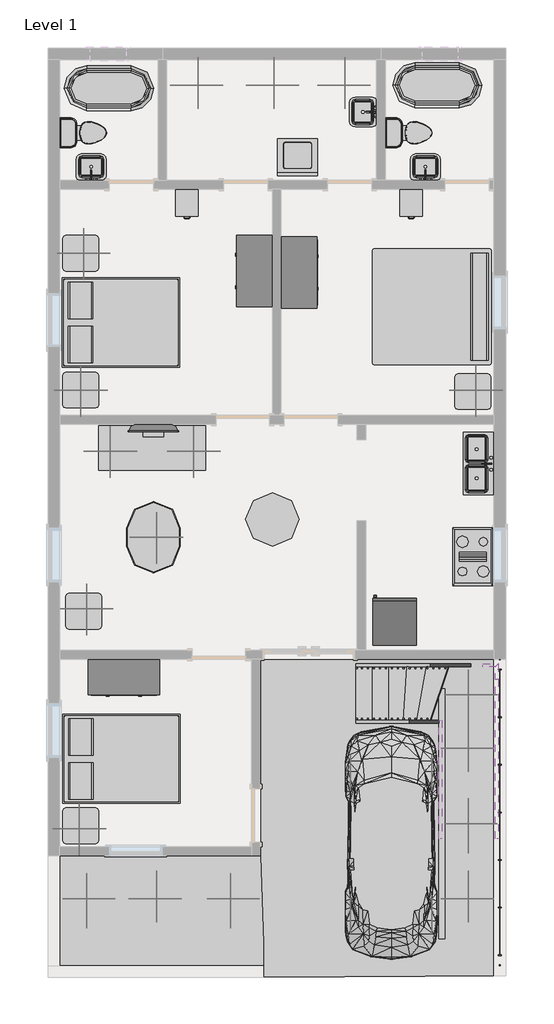
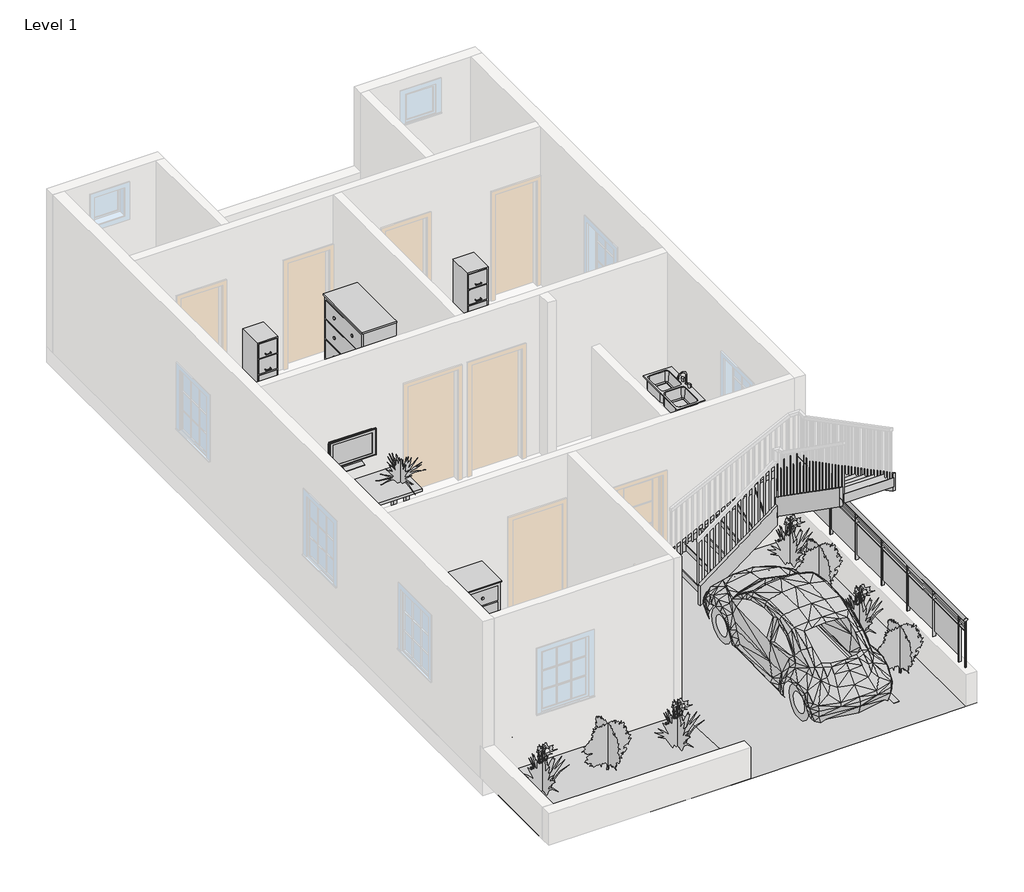
# One storey, part 3 of 3: 18 geographic elements, 17 furniture elements, 11 flow terminals, 7 proxies, 6 members, 1 railing, 1 stair flight.
"""IFC4 building model written with IfcOpenShell, lengths in millimetres."""

from ifc_helpers import new_model, si_unit, point, frame, origin, place, context, project, spatial, polyline, ellipse_curve, trimmed, outline, extrude, triangles, transform, mapped, element, save
from ifc_brep_helpers import plane_surface, extruded_surface, advanced_brep
from components import proxy_bb1e6e30, parking_space_9_x_18_90_deg_fdd9e8f5, rpc_beetle_rpc_beetle_3ce7ba48, proxy_a13a33b2, proxy_718fa39f, flow_terminal_accce45a, flow_terminal_a53be723, flow_terminal_62a433f7, toilet_domestic_3d_toilet_domestic_3d_f7549cf7, toilet_domestic_3d_toilet_domestic_3d_183bbd19, flow_terminal_b374fae2, furniture_1d2926bd, furniture_1fc5af50, furniture_552c1472, furniture_2babcf72, furniture_9fa109b2, furniture_56245f3a, furniture_be1c6672, furniture_905aceb5, furniture_31d08a24, furniture_62ce4b1f, rpc_plant_tropical_55f6ff97, rpc_plant_tropical_agave_1_5_93a2a214, rpc_plant_tropical_jungle_flame_3_9c4808c2, stair_flight_0e2f916f

model = new_model("IFC4")

# Units and contexts
model_context = context("Model", 3, world=origin())
ifc_project = project(units=[si_unit("LENGTHUNIT", "METRE", prefix="MILLI")], contexts=[model_context])

# Site, building, storey
site = spatial("IfcSite", under=ifc_project)
building = spatial("IfcBuilding", under=site)
storey = spatial("IfcBuildingStorey", under=building, Name="Level 1", Elevation=0.0)

# Proxies
placement = place(None, origin())
element("IfcBuildingElementProxy", 1, Name="Building Element Proxy", at=placement, inside=storey, context=model_context, shape_type="Tessellation", body=[
    triangles([(578.7339698, 220.6003974, 0.0), (4731.6338608, 239.6503974, 0.0), (4731.6338608, -4560.9495117, 0.0), (591.4339577, -4611.7496086, 0.0), (616.8340061, 322.2003914, 0.0), (540.6339698, -3113.1495117, 0.0), (540.6339698, 239.6503974, 0.0), (2115.4339577, 322.2003914, 0.0), (4731.6338608, -5170.5495117, 0.0), (591.4339577, -5195.9497055, 0.0)], [[10, 4, 6], [4, 10, 9], [7, 6, 1], [8, 1, 6], [7, 1, 5], [6, 4, 3], [3, 4, 9], [8, 6, 3], [8, 5, 1], [8, 3, 2]], closed=False),
])
element("IfcBuildingElementProxy", 2, Name="Building Element Proxy", at=placement, inside=storey, context=model_context, shape_type="Tessellation", body=[
    triangles([(-3091.5659454, -3113.1495117, 0.0), (-3091.5659454, -4611.7496086, 0.0), (540.6339698, -3113.1495117, 0.0), (591.4339577, -4611.7496086, 0.0), (591.4339577, -5195.9497055, 0.0), (-3091.5659454, -5195.9497055, 0.0)], [[4, 2, 5], [2, 6, 5], [1, 2, 3], [2, 4, 3]], closed=False),
])
proxy_shape = proxy_bb1e6e30(model_context)
element("IfcBuildingElementProxy", 3, Name="Cook Top-4 Unit : 36\" x 20\"", ObjectType="Cook Top-4 Unit : 36\" x 20\"", at=placement, inside=storey, context=model_context, shape_type="MappedRepresentation", body=[
    mapped(proxy_shape, transform((4172.8339716, 1992.250395, 0.0), x_axis=(0.0, -1.0000000000000004, 0.0), y_axis=(1.0000000000000004, 0.0, 0.0), z_axis=(0.0, 0.0, 1.0))),
])
parking_space_9_x_18_90_deg_shape = parking_space_9_x_18_90_deg_fdd9e8f5(model_context)
element("IfcBuildingElementProxy", 4, Name="Parking Space : 9' x 18' - 90 deg", ObjectType="Parking Space : 9' x 18' - 90 deg", at=placement, inside=storey, context=model_context, shape_type="MappedRepresentation", body=[
    mapped(parking_space_9_x_18_90_deg_shape, transform((3639.4339716, -4535.549605, 0.0), x_axis=(-1.0000000000000004, 0.0, 0.0), y_axis=(0.0, -1.0000000000000004, 0.0), z_axis=(0.0, 0.0, 1.0))),
])
rpc_beetle_rpc_beetle_shape = rpc_beetle_rpc_beetle_3ce7ba48(model_context)
element("IfcBuildingElementProxy", 5, Name="RPC Beetle : RPC Beetle", ObjectType="RPC Beetle : RPC Beetle", at=placement, inside=storey, context=model_context, shape_type="MappedRepresentation", body=[
    mapped(rpc_beetle_rpc_beetle_shape, transform((2775.8339716, -4129.149605, 0.0), x_axis=(1.0, 0.0, 0.0), y_axis=(0.0, 1.0, 0.0), z_axis=(0.0, 0.0, 1.0))),
])
proxy_2_shape = proxy_a13a33b2(model_context)
element("IfcBuildingElementProxy", 6, Name="Refrigerator : 30\" x 32\" RH", ObjectType="Refrigerator : 30\" x 32\" RH", at=placement, inside=storey, context=model_context, shape_type="MappedRepresentation", body=[
    mapped(proxy_2_shape, transform((2834.5714716, 867.1014235, 0.0), x_axis=(-1.0000000000000004, 0.0, 0.0), y_axis=(0.0, -1.0000000000000004, 0.0), z_axis=(0.0, 0.0, 1.0))),
])
proxy_3_shape = proxy_718fa39f(model_context)
element("IfcBuildingElementProxy", 7, Name="Washer : 27\" x 25\" x 35\"", ObjectType="Washer : 27\" x 25\" x 35\"", at=placement, inside=storey, context=model_context, shape_type="MappedRepresentation", body=[
    mapped(proxy_3_shape, transform((1594.7339716, 9091.8008302, 0.0), x_axis=(-1.0000000000000004, 0.0, 0.0), y_axis=(0.0, -1.0000000000000004, 0.0), z_axis=(0.0, 0.0, 1.0))),
])

# Flow terminals
flow_terminal_shape = flow_terminal_accce45a(model_context)
element("IfcFlowTerminal", 8, ObjectType="Floor Drain - Round : 5\" Strainer - 2\" Drain", at=placement, inside=storey, context=model_context, shape_type="MappedRepresentation", body=[
    mapped(flow_terminal_shape, transform((-1389.7660284, 9218.550395, 0.0), x_axis=(1.0, 0.0, 0.0), y_axis=(0.0, 1.0, 0.0), z_axis=(0.0, 0.0, 1.0))),
])
element("IfcFlowTerminal", 9, ObjectType="Floor Drain - Round : 5\" Strainer - 2\" Drain", at=placement, inside=storey, context=model_context, shape_type="MappedRepresentation", body=[
    mapped(flow_terminal_shape, transform((2166.2339716, 8932.800395, 0.0), x_axis=(1.0, 0.0, 0.0), y_axis=(0.0, 1.0, 0.0), z_axis=(0.0, 0.0, 1.0))),
])
element("IfcFlowTerminal", 10, ObjectType="Floor Drain - Round : 5\" Strainer - 2\" Drain", at=placement, inside=storey, context=model_context, shape_type="MappedRepresentation", body=[
    mapped(flow_terminal_shape, transform((4325.2339716, 9504.300395, 0.0), x_axis=(1.0, 0.0, 0.0), y_axis=(0.0, 1.0, 0.0), z_axis=(0.0, 0.0, 1.0))),
])
flow_terminal_2_shape = flow_terminal_a53be723(model_context)
element("IfcFlowTerminal", 11, ObjectType="Sink Kitchen-Double : 42\" x 21\"", at=placement, inside=storey, context=model_context, shape_type="MappedRepresentation", body=[
    mapped(flow_terminal_2_shape, transform((4272.0885705, 3595.4396356, 0.0), x_axis=(0.0, -1.0000000000000004, 0.0), y_axis=(1.0000000000000004, 0.0, 0.0), z_axis=(0.0, 0.0, 1.0))),
])
flow_terminal_3_shape = flow_terminal_62a433f7(model_context)
element("IfcFlowTerminal", 12, ObjectType="Sink Vanity-Square : 20\" x 18\"", at=placement, inside=storey, context=model_context, shape_type="MappedRepresentation", body=[
    mapped(flow_terminal_3_shape, transform((2341.6885705, 9602.5396356, 0.0), x_axis=(0.0, -1.0000000000000004, 0.0), y_axis=(1.0000000000000004, 0.0, 0.0), z_axis=(0.0, 0.0, 1.0))),
])
element("IfcFlowTerminal", 13, ObjectType="Sink Vanity-Square : 20\" x 18\"", at=placement, inside=storey, context=model_context, shape_type="MappedRepresentation", body=[
    mapped(flow_terminal_3_shape, transform((3375.7232122, 8598.5957961, 0.0), x_axis=(-1.0, 0.0, 0.0), y_axis=(0.0, -1.0, 0.0), z_axis=(0.0, 0.0, 1.0))),
])
element("IfcFlowTerminal", 14, ObjectType="Sink Vanity-Square : 20\" x 18\"", at=placement, inside=storey, context=model_context, shape_type="MappedRepresentation", body=[
    mapped(flow_terminal_3_shape, transform((-2339.2767878, 8598.5957961, 0.0), x_axis=(-1.0000000000000002, 0.0, 0.0), y_axis=(0.0, -1.0000000000000002, 0.0), z_axis=(0.0, 0.0, 1.0))),
])
toilet_domestic_3d_toilet_domestic_3d_shape = toilet_domestic_3d_toilet_domestic_3d_f7549cf7(model_context)
toilet_domestic_3d_toilet_domestic_3d_2_shape = toilet_domestic_3d_toilet_domestic_3d_183bbd19(model_context)
element("IfcFlowTerminal", 15, ObjectType="Toilet-Domestic-3D : Toilet-Domestic-3D", at=placement, inside=storey, context=model_context, shape_type="MappedRepresentation", body=[
    mapped(toilet_domestic_3d_toilet_domestic_3d_shape, transform((3168.929999, 9231.250395, 0.0), x_axis=(0.0, 1.0, 0.0), y_axis=(-1.0, 0.0, 0.0), z_axis=(0.0, 0.0, 1.0))),
    mapped(toilet_domestic_3d_toilet_domestic_3d_2_shape, transform((3168.929999, 9231.250395, 0.0), x_axis=(0.0, 1.0, 0.0), y_axis=(-1.0, 0.0, 0.0), z_axis=(0.0, 0.0, 1.0))),
])
element("IfcFlowTerminal", 16, ObjectType="Toilet-Domestic-3D : Toilet-Domestic-3D", at=placement, inside=storey, context=model_context, shape_type="MappedRepresentation", body=[
    mapped(toilet_domestic_3d_toilet_domestic_3d_shape, transform((-2393.670001, 9231.250395, 0.0), x_axis=(0.0, 1.0, 0.0), y_axis=(-1.0, 0.0, 0.0), z_axis=(0.0, 0.0, 1.0))),
    mapped(toilet_domestic_3d_toilet_domestic_3d_2_shape, transform((-2393.670001, 9231.250395, 0.0), x_axis=(0.0, 1.0, 0.0), y_axis=(-1.0, 0.0, 0.0), z_axis=(0.0, 0.0, 1.0))),
])
flow_terminal_4_shape = flow_terminal_b374fae2(model_context)
element("IfcFlowTerminal", 17, ObjectType="Tub-Free Standing-3D : 30\" x 60\"", at=placement, inside=storey, context=model_context, shape_type="MappedRepresentation", body=[
    mapped(flow_terminal_4_shape, transform((3563.2339716, 10044.050395, 0.0), x_axis=(0.0, 1.0, 0.0), y_axis=(-1.0, 0.0, 0.0), z_axis=(0.0, 0.0, 1.0))),
])
element("IfcFlowTerminal", 18, ObjectType="Tub-Free Standing-3D : 30\" x 60\"", at=placement, inside=storey, context=model_context, shape_type="MappedRepresentation", body=[
    mapped(flow_terminal_4_shape, transform((-2050.1660284, 9993.250395, 0.0), x_axis=(0.0, 1.0000000000000002, 0.0), y_axis=(-1.0000000000000002, 0.0, 0.0), z_axis=(0.0, 0.0, 1.0))),
])

# Furniture
furniture_shape = furniture_1d2926bd(model_context)
element("IfcFurniture", 19, ObjectType="Bed-Box : Queen 60\" x 79\"", at=placement, inside=storey, context=model_context, shape_type="MappedRepresentation", body=[
    mapped(furniture_shape, transform((-2081.3955366, 5653.597936, 0.0), x_axis=(0.0, 1.0, 0.0), y_axis=(-1.0, 0.0, 0.0), z_axis=(0.0, 0.0, 1.0))),
])
element("IfcFurniture", 20, ObjectType="Bed-Box : Queen 60\" x 79\"", at=placement, inside=storey, context=model_context, shape_type="MappedRepresentation", body=[
    mapped(furniture_shape, transform((-2068.6955366, -1801.302064, 0.0), x_axis=(0.0, 1.0, 0.0), y_axis=(-1.0, 0.0, 0.0), z_axis=(0.0, 0.0, 1.0))),
])
furniture_2_shape = furniture_1fc5af50(model_context)
element("IfcFurniture", 21, ObjectType="Bed-Standard.0001 : King 78\" x 80\"", at=placement, inside=storey, context=model_context, shape_type="MappedRepresentation", body=[
    mapped(furniture_2_shape, transform((3519.9290536, 6530.9389196, 0.0), x_axis=(0.0, -1.0, 0.0), y_axis=(1.0, 0.0, 0.0), z_axis=(0.0, 0.0, 1.0))),
])
furniture_3_shape = furniture_552c1472(model_context)
element("IfcFurniture", 22, ObjectType="Cabinet-File 3 Drawer : 15\" x 18\"", at=placement, inside=storey, context=model_context, shape_type="MappedRepresentation", body=[
    mapped(furniture_3_shape, transform((3246.6304187, 8179.5846951, 0.0), x_axis=(1.0, 0.0, 0.0), y_axis=(0.0, 1.0, 0.0), z_axis=(0.0, 0.0, 1.0))),
])
element("IfcFurniture", 23, ObjectType="Cabinet-File 3 Drawer : 15\" x 18\"", at=placement, inside=storey, context=model_context, shape_type="MappedRepresentation", body=[
    mapped(furniture_3_shape, transform((-588.7695813, 8179.5846951, 0.0), x_axis=(1.0, 0.0, 0.0), y_axis=(0.0, 1.0, 0.0), z_axis=(0.0, 0.0, 1.0))),
])
furniture_4_shape = furniture_2babcf72(model_context)
element("IfcFurniture", 24, ObjectType="Dresser : 48\" x 60\" x 24\"", at=placement, inside=storey, context=model_context, shape_type="MappedRepresentation", body=[
    mapped(furniture_4_shape, transform((-1526.9727685, 298.0133491, 0.0), x_axis=(1.0, 0.0, 0.0), y_axis=(0.0, 1.0, 0.0), z_axis=(0.0, 0.0, 1.0))),
])
furniture_5_shape = furniture_9fa109b2(model_context)
element("IfcFurniture", 25, ObjectType="Dresser : 48\" x 72\" x 24\"", at=placement, inside=storey, context=model_context, shape_type="MappedRepresentation", body=[
    mapped(furniture_5_shape, transform((802.1969257, 6599.8571352, 0.0), x_axis=(0.0, -1.0000000000000007, 0.0), y_axis=(1.0000000000000007, 0.0, 0.0), z_axis=(0.0, 0.0, 1.0))),
])
element("IfcFurniture", 26, ObjectType="Dresser : 48\" x 72\" x 24\"", at=placement, inside=storey, context=model_context, shape_type="MappedRepresentation", body=[
    mapped(furniture_5_shape, transform((837.8710175, 7112.8436548, 0.0), x_axis=(0.0, 1.0000000000000002, 0.0), y_axis=(-1.0000000000000002, 0.0, 0.0), z_axis=(0.0, 0.0, 1.0))),
])
furniture_6_shape = furniture_56245f3a(model_context)
element("IfcFurniture", 27, ObjectType="TV - Flat Screen : 32\"", at=placement, inside=storey, context=model_context, shape_type="MappedRepresentation", body=[
    mapped(furniture_6_shape, transform((-1284.2215142, 4194.3117714, 1041.4), x_axis=(1.0, 0.0, 0.0), y_axis=(0.0, 1.0, 0.0), z_axis=(0.0, 0.0, 1.0))),
])
furniture_7_shape = furniture_be1c6672(model_context)
element("IfcFurniture", 28, ObjectType="Table-Dining Oval : 36\" x 48\"", at=placement, inside=storey, context=model_context, shape_type="MappedRepresentation", body=[
    mapped(furniture_7_shape, transform((-1646.264389, 2724.2700671, 0.0), x_axis=(0.0, 1.0, 0.0), y_axis=(-1.0, 0.0, 0.0), z_axis=(0.0, 0.0, 1.0))),
])
furniture_8_shape = furniture_905aceb5(model_context)
element("IfcFurniture", 29, ObjectType="Table-Dining Round w Chairs : 36\" Diameter", at=placement, inside=storey, context=model_context, shape_type="MappedRepresentation", body=[
    mapped(furniture_8_shape, transform((640.1520044, 2812.1290835, 0.0), x_axis=(1.0, 0.0, 0.0), y_axis=(0.0, 1.0, 0.0), z_axis=(0.0, 0.0, 1.0))),
])
furniture_9_shape = furniture_31d08a24(model_context)
element("IfcFurniture", 30, ObjectType="Table-End : 24\" x 24\"", at=placement, inside=storey, context=model_context, shape_type="MappedRepresentation", body=[
    mapped(furniture_9_shape, transform((-2841.2996587, 7021.450395, 0.0), x_axis=(1.0, 0.0, 0.0), y_axis=(0.0, 1.0, 0.0), z_axis=(0.0, 0.0, 1.0))),
])
element("IfcFurniture", 31, ObjectType="Table-End : 24\" x 24\"", at=placement, inside=storey, context=model_context, shape_type="MappedRepresentation", body=[
    mapped(furniture_9_shape, transform((-2841.2996587, 4684.650395, 0.0), x_axis=(1.0, 0.0, 0.0), y_axis=(0.0, 1.0, 0.0), z_axis=(0.0, 0.0, 1.0))),
])
element("IfcFurniture", 32, ObjectType="Table-End : 24\" x 24\"", at=placement, inside=storey, context=model_context, shape_type="MappedRepresentation", body=[
    mapped(furniture_9_shape, transform((3864.3003413, 4659.250395, 0.0), x_axis=(1.0, 0.0, 0.0), y_axis=(0.0, 1.0, 0.0), z_axis=(0.0, 0.0, 1.0))),
])
element("IfcFurniture", 33, ObjectType="Table-End : 24\" x 24\"", at=placement, inside=storey, context=model_context, shape_type="MappedRepresentation", body=[
    mapped(furniture_9_shape, transform((-2790.4996587, 906.400395, 0.0), x_axis=(1.0, 0.0, 0.0), y_axis=(0.0, 1.0, 0.0), z_axis=(0.0, 0.0, 1.0))),
])
element("IfcFurniture", 34, ObjectType="Table-End : 24\" x 24\"", at=placement, inside=storey, context=model_context, shape_type="MappedRepresentation", body=[
    mapped(furniture_9_shape, transform((-2841.2996587, -2757.549605, 0.0), x_axis=(1.0, 0.0, 0.0), y_axis=(0.0, 1.0, 0.0), z_axis=(0.0, 0.0, 1.0))),
])
furniture_10_shape = furniture_62ce4b1f(model_context)
element("IfcFurniture", 35, ObjectType="Table-Rectangular : 72\" x 30\"", at=placement, inside=storey, context=model_context, shape_type="MappedRepresentation", body=[
    mapped(furniture_10_shape, transform((-1313.5660284, 3846.450395, 0.0), x_axis=(1.0, 0.0, 0.0), y_axis=(0.0, 1.0, 0.0), z_axis=(0.0, 0.0, 1.0))),
])

# Geographic elements
rpc_plant_tropical_shape = rpc_plant_tropical_55f6ff97(model_context)
element("IfcGeographicElement", 36, ObjectType="RPC Plant - Tropical", at=placement, inside=storey, context=model_context, shape_type="MappedRepresentation", body=[
    mapped(rpc_plant_tropical_shape, transform((-2431.1660284, -3849.749605, 0.0), x_axis=(1.0, 0.0, 0.0), y_axis=(0.0, 1.0, 0.0), z_axis=(0.0, 0.0, 1.0))),
])
element("IfcGeographicElement", 37, ObjectType="RPC Plant - Tropical", at=placement, inside=storey, context=model_context, shape_type="MappedRepresentation", body=[
    mapped(rpc_plant_tropical_shape, transform((32.6339716, -3849.749605, 0.0), x_axis=(1.0, 0.0, 0.0), y_axis=(0.0, 1.0, 0.0), z_axis=(0.0, 0.0, 1.0))),
])
element("IfcGeographicElement", 38, ObjectType="RPC Plant - Tropical", at=placement, inside=storey, context=model_context, shape_type="MappedRepresentation", body=[
    mapped(rpc_plant_tropical_shape, transform((4096.6339716, -369.949605, 0.0), x_axis=(1.0, 0.0, 0.0), y_axis=(0.0, 1.0, 0.0), z_axis=(0.0, 0.0, 1.0))),
])
element("IfcGeographicElement", 39, ObjectType="RPC Plant - Tropical", at=placement, inside=storey, context=model_context, shape_type="MappedRepresentation", body=[
    mapped(rpc_plant_tropical_shape, transform((4096.6339716, -2569.2865945, 0.0), x_axis=(1.0, 0.0, 0.0), y_axis=(0.0, 1.0, 0.0), z_axis=(0.0, 0.0, 1.0))),
])
rpc_plant_tropical_agave_1_5_shape = rpc_plant_tropical_agave_1_5_93a2a214(model_context)
element("IfcGeographicElement", 40, ObjectType="RPC Plant - Tropical : Agave - 1.5'", at=placement, inside=storey, context=model_context, shape_type="MappedRepresentation", body=[
    mapped(rpc_plant_tropical_agave_1_5_shape, transform((-2481.9660284, 7173.850395, 609.6), x_axis=(1.0, 0.0, 0.0), y_axis=(0.0, 1.0, 0.0), z_axis=(0.0, 0.0, 1.0))),
])
element("IfcGeographicElement", 41, ObjectType="RPC Plant - Tropical : Agave - 1.5'", at=placement, inside=storey, context=model_context, shape_type="MappedRepresentation", body=[
    mapped(rpc_plant_tropical_agave_1_5_shape, transform((-2532.7660284, 4837.050395, 609.6), x_axis=(1.0, 0.0, 0.0), y_axis=(0.0, 1.0, 0.0), z_axis=(0.0, 0.0, 1.0))),
])
element("IfcGeographicElement", 42, ObjectType="RPC Plant - Tropical : Agave - 1.5'", at=placement, inside=storey, context=model_context, shape_type="MappedRepresentation", body=[
    mapped(rpc_plant_tropical_agave_1_5_shape, transform((4223.6339716, 4837.050395, 609.6), x_axis=(1.0, 0.0, 0.0), y_axis=(0.0, 1.0, 0.0), z_axis=(0.0, 0.0, 1.0))),
])
element("IfcGeographicElement", 43, ObjectType="RPC Plant - Tropical : Agave - 1.5'", at=placement, inside=storey, context=model_context, shape_type="MappedRepresentation", body=[
    mapped(rpc_plant_tropical_agave_1_5_shape, transform((-2431.1660284, 1103.250395, 609.6), x_axis=(1.0, 0.0, 0.0), y_axis=(0.0, 1.0, 0.0), z_axis=(0.0, 0.0, 1.0))),
])
element("IfcGeographicElement", 44, ObjectType="RPC Plant - Tropical : Agave - 1.5'", at=placement, inside=storey, context=model_context, shape_type="MappedRepresentation", body=[
    mapped(rpc_plant_tropical_agave_1_5_shape, transform((-1237.3660284, 2322.450395, 609.6), x_axis=(1.0, 0.0, 0.0), y_axis=(0.0, 1.0, 0.0), z_axis=(0.0, 0.0, 1.0))),
])
element("IfcGeographicElement", 45, ObjectType="RPC Plant - Tropical : Agave - 1.5'", at=placement, inside=storey, context=model_context, shape_type="MappedRepresentation", body=[
    mapped(rpc_plant_tropical_agave_1_5_shape, transform((-2024.7660284, 3795.650395, 685.8), x_axis=(1.0, 0.0, 0.0), y_axis=(0.0, 1.0, 0.0), z_axis=(0.0, 0.0, 1.0))),
])
element("IfcGeographicElement", 46, ObjectType="RPC Plant - Tropical : Agave - 1.5'", at=placement, inside=storey, context=model_context, shape_type="MappedRepresentation", body=[
    mapped(rpc_plant_tropical_agave_1_5_shape, transform((-602.3660284, 3795.650395, 685.8), x_axis=(1.0, 0.0, 0.0), y_axis=(0.0, 1.0, 0.0), z_axis=(0.0, 0.0, 1.0))),
])
element("IfcGeographicElement", 47, ObjectType="RPC Plant - Tropical : Agave - 1.5'", at=placement, inside=storey, context=model_context, shape_type="MappedRepresentation", body=[
    mapped(rpc_plant_tropical_agave_1_5_shape, transform((-2558.1660284, -2655.949605, 609.6), x_axis=(1.0, 0.0, 0.0), y_axis=(0.0, 1.0, 0.0), z_axis=(0.0, 0.0, 1.0))),
])
rpc_plant_tropical_jungle_flame_3_shape = rpc_plant_tropical_jungle_flame_3_9c4808c2(model_context)
element("IfcGeographicElement", 48, ObjectType="RPC Plant - Tropical : Jungle Flame - 3'", at=placement, inside=storey, context=model_context, shape_type="MappedRepresentation", body=[
    mapped(rpc_plant_tropical_jungle_flame_3_shape, transform((-526.1660284, 10044.050395, 0.0), x_axis=(1.0, 0.0, 0.0), y_axis=(0.0, 1.0, 0.0), z_axis=(0.0, 0.0, 1.0))),
])
element("IfcGeographicElement", 49, ObjectType="RPC Plant - Tropical : Jungle Flame - 3'", at=placement, inside=storey, context=model_context, shape_type="MappedRepresentation", body=[
    mapped(rpc_plant_tropical_jungle_flame_3_shape, transform((769.2339716, 10044.050395, 0.0), x_axis=(1.0, 0.0, 0.0), y_axis=(0.0, 1.0, 0.0), z_axis=(0.0, 0.0, 1.0))),
])
element("IfcGeographicElement", 50, ObjectType="RPC Plant - Tropical : Jungle Flame - 3'", at=placement, inside=storey, context=model_context, shape_type="MappedRepresentation", body=[
    mapped(rpc_plant_tropical_jungle_flame_3_shape, transform((1988.4339716, 10044.050395, 0.0), x_axis=(1.0, 0.0, 0.0), y_axis=(0.0, 1.0, 0.0), z_axis=(0.0, 0.0, 1.0))),
])
element("IfcGeographicElement", 51, ObjectType="RPC Plant - Tropical : Jungle Flame - 3'", at=placement, inside=storey, context=model_context, shape_type="MappedRepresentation", body=[
    mapped(rpc_plant_tropical_jungle_flame_3_shape, transform((-1237.3660284, -3849.749605, 0.0), x_axis=(1.0, 0.0, 0.0), y_axis=(0.0, 1.0, 0.0), z_axis=(0.0, 0.0, 1.0))),
])
element("IfcGeographicElement", 52, ObjectType="RPC Plant - Tropical : Jungle Flame - 3'", at=placement, inside=storey, context=model_context, shape_type="MappedRepresentation", body=[
    mapped(rpc_plant_tropical_jungle_flame_3_shape, transform((4096.6339716, -1284.349605, 0.0), x_axis=(1.0, 0.0, 0.0), y_axis=(0.0, 1.0, 0.0), z_axis=(0.0, 0.0, 1.0))),
])
element("IfcGeographicElement", 53, ObjectType="RPC Plant - Tropical : Jungle Flame - 3'", at=placement, inside=storey, context=model_context, shape_type="MappedRepresentation", body=[
    mapped(rpc_plant_tropical_jungle_flame_3_shape, transform((4096.6339716, -3849.749605, 0.0), x_axis=(1.0, 0.0, 0.0), y_axis=(0.0, 1.0, 0.0), z_axis=(0.0, 0.0, 1.0))),
])

# Members
element("IfcMember", 54, ObjectType="Stringer - 2\" Width", at=placement, inside=storey, context=model_context, shape_type="SweptSolid", body=[
    extrude(outline(polyline([(572.8128502, 2176.6969821), (232.9712892, 2176.6969821), (1302.0770504, 4344.8241925), (1641.9186114, 4344.8241925), (572.8128502, 2176.6969821)])), frame((0.0, 112.650395, 0.0), z_axis=(0.0, 1.0, 0.0), x_axis=(0.0, 0.0, 1.0)), (0.0, 0.0, 1.0), 50.8),
])
element("IfcMember", 55, ObjectType="Stringer - 2\" Width", at=placement, inside=storey, context=model_context, shape_type="SweptSolid", body=[
    extrude(outline(polyline([(4344.8241925, 112.650395), (4344.8241925, 163.450395), (4604.6339716, 163.450395), (4553.8339716, 112.650395), (4344.8241925, 112.650395)])), frame((0.0, 0.0, 1302.0770504), z_axis=(0.0, 0.0, 1.0), x_axis=(1.0, 0.0, 0.0)), (0.0, 0.0, 1.0), 339.8415609),
])
element("IfcMember", 56, ObjectType="Stringer - 2\" Width", at=placement, inside=storey, context=model_context, shape_type="SweptSolid", body=[
    extrude(outline(polyline([(4553.8339716, 112.650395), (4604.6339716, 163.450395), (4604.6339716, -105.5029481), (4553.8339716, -105.5029481), (4553.8339716, 112.650395)])), frame((0.0, 0.0, 1302.0770504), z_axis=(0.0, 0.0, 1.0), x_axis=(1.0, 0.0, 0.0)), (0.0, 0.0, 1.0), 339.8415609),
])
element("IfcMember", 57, ObjectType="Stringer - 2\" Width", at=placement, inside=storey, context=model_context, shape_type="SweptSolid", body=[
    extrude(outline(polyline([(-105.5029481, 1641.9186114), (-105.5029481, 1302.0770504), (-2823.2865945, 2717.5988597), (-2823.2865945, 3057.4404207), (-105.5029481, 1641.9186114)])), frame((4553.8339716, 0.0, 0.0), z_axis=(1.0, 0.0, 0.0), x_axis=(0.0, 1.0, 0.0)), (0.0, 0.0, 1.0), 50.8),
])
element("IfcMember", 58, ObjectType="Stringer - 2\" Width", at=placement, inside=storey, context=model_context, shape_type="SweptSolid", body=[
    extrude(outline(polyline([(525.8525026, 2176.6969821), (145.2804064, 2176.6969821), (1200.9261811, 3588.6339716), (1581.4982774, 3588.6339716), (525.8525026, 2176.6969821)])), frame((0.0, -852.549605, 0.0), z_axis=(0.0, 1.0, 0.0), x_axis=(0.0, 0.0, 1.0)), (0.0, 0.0, 1.0), 50.8),
])
element("IfcMember", 59, ObjectType="Stringer - 2\" Width", at=placement, inside=storey, context=model_context, shape_type="SweptSolid", body=[
    extrude(outline(polyline([(-801.749605, 1709.9296678), (-801.749605, 1337.7212805), (-2823.2865945, 2754.5609981), (-2823.2865945, 3126.7693854), (-801.749605, 1709.9296678)])), frame((3588.6339716, 0.0, 0.0), z_axis=(1.0, 0.0, 0.0), x_axis=(0.0, 1.0, 0.0)), (0.0, 0.0, 1.0), 50.8),
])

# Railing
element("IfcRailing", 60, ObjectType="Glass Panel - Bottom Fill", at=placement, inside=storey, context=model_context, shape_type="SolidModel", body=[
    advanced_brep(
    [(4668.1339716, 239.650395, 1524.0), (4591.9339716, 239.650395, 1524.0), (4668.1339716, -4992.749605, 1524.0), (4591.9339716, -4992.749605, 1524.0)],
    [
        (0, 1, ellipse_curve(frame((4630.0339716, 239.650395, 1524.0), z_axis=(0.0, 1.0, 0.0), x_axis=(-1.0, 0.0, 0.0)), 38.1, 28.575)),
        (1, 0, ellipse_curve(frame((4630.0339716, 239.650395, 1524.0), z_axis=(0.0, 1.0, 0.0), x_axis=(-1.0, 0.0, 0.0)), 38.1, 28.575)),
        (2, 3, ellipse_curve(frame((4630.0339716, -4992.749605, 1524.0), z_axis=(0.0, -1.0, 0.0), x_axis=(-1.0, 0.0, 0.0)), 38.1, 28.575)),
        (3, 2, ellipse_curve(frame((4630.0339716, -4992.749605, 1524.0), z_axis=(0.0, -1.0, 0.0), x_axis=(-1.0, 0.0, 0.0)), 38.1, 28.575)),
        (0, 2),
        (3, 1),
    ],
    [
        plane_surface(frame((4630.0339716, 239.650395, 1524.0), z_axis=(0.0, 1.0, 0.0), x_axis=(0.0, 0.0, -1.0))),
        plane_surface(frame((4630.0339716, -4992.749605, 1524.0), z_axis=(0.0, -1.0, 0.0), x_axis=(0.0, 0.0, -1.0))),
        extruded_surface(trimmed(ellipse_curve(frame((4630.0339716, -4992.749605, 1524.0), z_axis=(0.0, 1.0, 0.0), x_axis=(-1.0, 0.0, 0.0)), 38.1, 28.575), [point((4668.1339716, -4992.749605, 1524.0))], [point((4591.9339716, -4992.749605, 1524.0))], True, "CARTESIAN"), (0.0, 5232.4, 0.0), 5232.4),
        extruded_surface(trimmed(ellipse_curve(frame((4630.0339716, -4992.749605, 1524.0), z_axis=(0.0, 1.0, 0.0), x_axis=(-1.0, 0.0, 0.0)), 38.1, 28.575), [point((4591.9339716, -4992.749605, 1524.0))], [point((4668.1339716, -4992.749605, 1524.0))], True, "CARTESIAN"), (0.0, 5232.4, 0.0), 5232.4),
    ],
    [
        (0, [[1, 2]]),
        (1, [[3, 4]]),
        (2, [[-1, 5, -4, 6]]),
        (3, [[-2, -6, -3, -5]]),
    ],
),
    extrude(outline(polyline([(4617.3339716, 239.650395), (4642.7339716, 239.650395), (4642.7339716, -4992.749605), (4617.3339716, -4992.749605), (4617.3339716, 239.650395)])), frame((0.0, 0.0, 1409.7), z_axis=(0.0, 0.0, 1.0), x_axis=(1.0, 0.0, 0.0)), (0.0, 0.0, 1.0), 25.4),
    extrude(outline(polyline([(4617.3339716, 239.650395), (4642.7339716, 239.650395), (4642.7339716, -4992.749605), (4617.3339716, -4992.749605), (4617.3339716, 239.650395)])), frame((0.0, 0.0, 1308.1), z_axis=(0.0, 0.0, 1.0), x_axis=(1.0, 0.0, 0.0)), (0.0, 0.0, 1.0), 25.4),
    extrude(outline(polyline([(4604.6339716, -4808.599605), (4655.4339716, -4808.599605), (4655.4339716, -4821.299605), (4604.6339716, -4821.299605), (4604.6339716, -4808.599605)])), frame((0.0, 0.0, 609.6), z_axis=(0.0, 0.0, 1.0), x_axis=(1.0, 0.0, 0.0)), (0.0, 0.0, 1.0), 885.6788223),
    extrude(outline(polyline([(4636.5691286, -4002.149605), (4636.5691286, -4814.949605), (4630.2191286, -4814.949605), (4630.2191286, -4002.149605), (4636.5691286, -4002.149605)])), frame((0.0, 0.0, 711.2), z_axis=(0.0, 0.0, 1.0), x_axis=(1.0, 0.0, 0.0)), (0.0, 0.0, 1.0), 596.9),
    extrude(outline(polyline([(4604.6339716, -3995.799605), (4655.4339716, -3995.799605), (4655.4339716, -4008.499605), (4604.6339716, -4008.499605), (4604.6339716, -3995.799605)])), frame((0.0, 0.0, 609.6), z_axis=(0.0, 0.0, 1.0), x_axis=(1.0, 0.0, 0.0)), (0.0, 0.0, 1.0), 885.6788223),
    extrude(outline(polyline([(4636.5691286, -3189.349605), (4636.5691286, -4002.149605), (4630.2191286, -4002.149605), (4630.2191286, -3189.349605), (4636.5691286, -3189.349605)])), frame((0.0, 0.0, 711.2), z_axis=(0.0, 0.0, 1.0), x_axis=(1.0, 0.0, 0.0)), (0.0, 0.0, 1.0), 596.9),
    extrude(outline(polyline([(4604.6339716, -3182.999605), (4655.4339716, -3182.999605), (4655.4339716, -3195.699605), (4604.6339716, -3195.699605), (4604.6339716, -3182.999605)])), frame((0.0, 0.0, 609.6), z_axis=(0.0, 0.0, 1.0), x_axis=(1.0, 0.0, 0.0)), (0.0, 0.0, 1.0), 885.6788223),
    extrude(outline(polyline([(4636.5691286, -2376.549605), (4636.5691286, -3189.349605), (4630.2191286, -3189.349605), (4630.2191286, -2376.549605), (4636.5691286, -2376.549605)])), frame((0.0, 0.0, 711.2), z_axis=(0.0, 0.0, 1.0), x_axis=(1.0, 0.0, 0.0)), (0.0, 0.0, 1.0), 596.9),
    extrude(outline(polyline([(4604.6339716, -2370.199605), (4655.4339716, -2370.199605), (4655.4339716, -2382.899605), (4604.6339716, -2382.899605), (4604.6339716, -2370.199605)])), frame((0.0, 0.0, 609.6), z_axis=(0.0, 0.0, 1.0), x_axis=(1.0, 0.0, 0.0)), (0.0, 0.0, 1.0), 885.6788223),
    extrude(outline(polyline([(4636.5691286, -1563.749605), (4636.5691286, -2376.549605), (4630.2191286, -2376.549605), (4630.2191286, -1563.749605), (4636.5691286, -1563.749605)])), frame((0.0, 0.0, 711.2), z_axis=(0.0, 0.0, 1.0), x_axis=(1.0, 0.0, 0.0)), (0.0, 0.0, 1.0), 596.9),
    extrude(outline(polyline([(4604.6339716, -1557.399605), (4655.4339716, -1557.399605), (4655.4339716, -1570.099605), (4604.6339716, -1570.099605), (4604.6339716, -1557.399605)])), frame((0.0, 0.0, 609.6), z_axis=(0.0, 0.0, 1.0), x_axis=(1.0, 0.0, 0.0)), (0.0, 0.0, 1.0), 885.6788223),
    extrude(outline(polyline([(4636.5691286, -750.949605), (4636.5691286, -1563.749605), (4630.2191286, -1563.749605), (4630.2191286, -750.949605), (4636.5691286, -750.949605)])), frame((0.0, 0.0, 711.2), z_axis=(0.0, 0.0, 1.0), x_axis=(1.0, 0.0, 0.0)), (0.0, 0.0, 1.0), 596.9),
    extrude(outline(polyline([(4604.6339716, -744.599605), (4655.4339716, -744.599605), (4655.4339716, -757.299605), (4604.6339716, -757.299605), (4604.6339716, -744.599605)])), frame((0.0, 0.0, 609.6), z_axis=(0.0, 0.0, 1.0), x_axis=(1.0, 0.0, 0.0)), (0.0, 0.0, 1.0), 885.6788223),
    extrude(outline(polyline([(4636.5691286, 61.850395), (4636.5691286, -750.949605), (4630.2191286, -750.949605), (4630.2191286, 61.850395), (4636.5691286, 61.850395)])), frame((0.0, 0.0, 711.2), z_axis=(0.0, 0.0, 1.0), x_axis=(1.0, 0.0, 0.0)), (0.0, 0.0, 1.0), 596.9),
    extrude(outline(polyline([(4604.6339716, 68.200395), (4655.4339716, 68.200395), (4655.4339716, 55.500395), (4604.6339716, 55.500395), (4604.6339716, 68.200395)])), frame((0.0, 0.0, 609.6), z_axis=(0.0, 0.0, 1.0), x_axis=(1.0, 0.0, 0.0)), (0.0, 0.0, 1.0), 885.6788223),
    extrude(outline(polyline([(4620.5089716, -4980.049605), (4639.5589716, -4980.049605), (4639.5589716, -4999.099605), (4620.5089716, -4999.099605), (4620.5089716, -4980.049605)])), frame((0.0, 0.0, 609.6), z_axis=(0.0, 0.0, 1.0), x_axis=(1.0, 0.0, 0.0)), (0.0, 0.0, 1.0), 885.6788223),
    extrude(outline(polyline([(4620.5089716, 246.000395), (4639.5589716, 246.000395), (4639.5589716, 226.950395), (4620.5089716, 226.950395), (4620.5089716, 246.000395)])), frame((0.0, 0.0, 609.6), z_axis=(0.0, 0.0, 1.0), x_axis=(1.0, 0.0, 0.0)), (0.0, 0.0, 1.0), 885.6788223),
])

# Stair flight
stair_flight_shape = stair_flight_0e2f916f(model_context)
element("IfcStairFlight", 61, ObjectType="2\" Tread 1\" Nosing 1/4\" Riser", at=placement, inside=storey, context=model_context, shape_type="MappedRepresentation", body=[
    mapped(stair_flight_shape, transform((0.0, 0.0, 0.0), x_axis=(1.0, 0.0, 0.0), y_axis=(0.0, 1.0, 0.0), z_axis=(0.0, 0.0, 1.0))),
])

save(model, "model.ifc")

# Revit data of these elements
# Type "Cook Top-4 Unit : 36\" x 20\""
#   Assembly Code = "E1090400"
#   Depth = 2' - 0"
#   Width = 3' - 0"
#   Burner Material = Steel, Chrome Plated
#   Cooktop Material = Steel, Polished
#   Default Elevation = 0
# Type "Parking Space : 9' x 18' - 90 deg"
#   Angle = 90.00°
#   Parking Length = 18' - 0"
#   Parking Width = 9' - 0"
#   pl = 14' - 0"
#   pw = 6' - 5"
# Type "RPC Beetle : RPC Beetle"
#   built-in parameter 1005195 = "RPC-16-0U6E-L4EG-ENH1-J3KF-SVEL-0TX4-C0"
#   Height = 0
# Type "Refrigerator : 30\" x 32\" RH"
#   Label = "REF."
#   Assembly Code = "E1090400"
#   Depth = 2' - 7 3/4"
#   Handle = 2' - 3"
#   Height = 5' - 10"
#   Rear Clearance = 0' - 2"
#   Top Door Height = 1' - 8"
#   Width = 2' - 5 3/8"
#   Material = Steel, Paint Finish, Ivory, Glossy
#   Default Elevation = 0
# Type "Washer : 27\" x 25\" x 35\""
#   Label = "W"
#   Assembly Code = "E1090400"
#   Depth = 2' - 1"
#   Height = 2' - 11"
#   Width = 2' - 3"
#   Washer Material = Steel, Paint Finish, Ivory, Matte
#   Default Elevation = 0
# Type "Floor Drain - Round : 5\" Strainer - 2\" Drain"
#   WFU = 2
#   Strainer Height = 0' - 3 1/4"
#   Strainer Radius = 0' - 2 1/2"
#   Strainer Diameter = 0' - 5"
#   Radius 6 = 0' - 0 5/8"
#   Radius 5 = 0' - 1 1/4"
#   Radius 4 = 0' - 1 7/8"
#   Radius 2 = 0' - 3.04167"
#   Radius 1 = 0' - 2.02083"
#   Radius 3 = 0' - 2 1/32"
#   Pipe Radius = 1"
#   Pipe Diameter = 2"
#   Height 2 = 0' - 0.725"
#   Height 1 = 0' - 1 13/16"
#   Body Radius = 0' - 4 1/16"
#   Body Height = 0' - 3 5/8"
#   Body Diameter = 0' - 8 1/8"
#   Drain Material = none
#   HWFU = 0
#   Default Elevation = 0
#   CWFU = 0
# Type "Sink Kitchen-Double : 42\" x 21\""
#   Assembly Code = "D2010410"
#   Counter Height = 3' - 0"
#   Depth = 1' - 9"
#   Width = 3' - 6"
#   Faucet Material = Steel, Polished
#   Sink Material = Steel, Polished
#   Default Elevation = 0
# Type "Sink Vanity-Square : 20\" x 18\""
#   Assembly Code = "D2010400"
#   Counter Height = 2' - 7"
#   Depth = 1' - 6"
#   Width = 1' - 8"
#   Basin Material = Porcelain, Linen
#   Faucet Material = Steel, Polished
#   Default Elevation = 0
# Type "Toilet-Domestic-3D : Toilet-Domestic-3D"
#   Assembly Code = "D2010110"
#   Toilet - Bowl/Basin Material = Porcelain, Linen
#   Toilet - Seat Material = Laminate, Linen, Matte
#   Default Elevation = 0
# Type "Tub-Free Standing-3D : 30\" x 60\""
#   Assembly Code = "D2010110"
#   Height = 1' - 6"
#   Length = 5' - 0"
#   Width = 2' - 6"
#   Tub Material = Porcelain, Ivory
#   Default Elevation = 0
# Type "Bed-Box : Queen 60\" x 79\""
#   Assembly Code = "E2020200"
#   Length = 6' - 7"
#   Width = 5' - 0"
#   Frame Material = Birch
#   Mattress Material = Linen, White
#   Default Elevation = 0
# Type "Bed-Standard.0001 : King 78\" x 80\""
#   Assembly Code = "E2020200"
#   Length = 6' - 8"
#   Width = 6' - 6"
#   Leg Material = Steel, Chrome Plated
#   Mattress Material = Linen, White
#   Default Elevation = 0
# Type "Cabinet-File 3 Drawer : 15\" x 18\""
#   Assembly Code = "E2020200"
#   Depth = 1' - 6"
#   Height = 3' - 5"
#   Width = 1' - 3"
#   Cabinet Material = Steel, Paint Finish, Ivory, Glossy
#   Handle Material = Steel, Chrome Plated
#   Default Elevation = 0
# Type "Dresser : 48\" x 60\" x 24\""
#   Assembly Code = "E2020200"
#   Depth = 2' - 0"
#   Height = 5' - 0"
#   Width = 4' - 0"
#   Dresser Material = Laminate - Ivory, Glossy
#   Drawer Material = Laminate, Ivory, Matte
#   Knob Material = Cherry
#   Default Elevation = 0
# Type "Dresser : 48\" x 72\" x 24\""
#   Assembly Code = "E2020200"
#   Depth = 2' - 0"
#   Height = 6' - 0"
#   Width = 4' - 0"
#   Dresser Material = Laminate - Ivory, Glossy
#   Drawer Material = Laminate, Ivory, Matte
#   Knob Material = Cherry
#   Default Elevation = 0
# Type "TV - Flat Screen : 32\""
#   SinAng = 0' - 0.0193"
#   L = 2' - 3.79372"
#   H = 1' - 3.6354"
#   Thickness = 0' - 4.33071"
#   Diagonal = 2' - 7.88976"
#   CosAng = 0' - 0.03431"
#   Stand [instance default] = yes
#   Default Elevation = 0
# Type "Table-Dining Oval : 36\" x 48\""
#   Assembly Code = "E2020200"
#   Length = 4' - 0"
#   Width = 3' - 0"
#   Base Material = Steel, Chrome Plated
#   Top Material = Glass - Clear, Grey
#   Default Elevation = 0
#   Description = (empty or 0)
# Type "Table-Dining Round w Chairs : 36\" Diameter"
#   Assembly Code = "E2020200"
#   Radius = 1' - 6"
#   Diameter = 3' - 0"
#   Height = 2' - 6"
#   Chairs = 4
#   Base Material = Pine
#   Top Material = Laminate, Linen, Matte
#   Default Elevation = 0
# Type "Table-End : 24\" x 24\""
#   Assembly Code = "E2020200"
#   Height = 2' - 0"
#   Length = 2' - 0"
#   Width = 2' - 0"
#   Base Material = Birch
#   Top Material = Laminate, Ivory, Matte
#   Default Elevation = 0
# Type "Table-Rectangular : 72\" x 30\""
#   Assembly Code = "E2020200"
#   Height = 2' - 3"
#   Length = 6' - 0"
#   Width = 2' - 6"
#   Base Material = Birch
#   Top Material = Birch
#   Default Elevation = 0
# Type "RPC Plant - Tropical"
#   built-in parameter 1005198 = "{2, 15},{39, RPC-16-FWM5-GM7X-C67P-4000-ST1L-LVER-AU},{1, 0},{1, 0},{2, 13},{1, 8},{5, Color},{1, 0},{1, 0},{3, 0.8},{3, 0.8},{3, 0.8},{1, 8},{7, BBoxMin},{1, 0},{1, 0},{1, 0},{1, 0},{1, 0},{1, 8},{7, BBoxMax},{1, 0},{1, 0},{1, 0},{1, 0},{1, 0},{2, 11},{9, RPCTypeId},{1, 0},{1, 0},{39, RPC-16-FWM5-GM7X-C67P-4000-ST1L-LVER-AU},{1, 6},{14, RPCPlantHeight},{1, 0},{1, 0},{1, 3},{2, 11},{7, keyword},{1, 0},{1, 0},{35, :RPCs:Shrubs [General]:Geometry:RPC},{2, 11},{8, category},{1, 0},{1, 0},{16, Shrubs [General]},{2, 11},{12, LocalizedUID},{1, 0},{1, 0},{10, Crane Lily},{2, 14},{6, Height},{1, 0},{1, 0},{1, 3},{1, 2},{16, Cast Reflections},{1, 0},{1, 0},{1, 0},{1, 2},{12, Cast Shadows},{1, 0},{1, 0},{1, 1},{1, 2},{9, Lock View},{1, 0},{1, 0},{1, 0},{1, 4},{5, ViewC},{1, 0},{1, 0},{1, 0},{21, assetlibrary_base.fbx},{1, 5},"
#   built-in parameter 1005195 = "RPC-16-FWM5-GM7X-C67P-4000-ST1L-LVER-AU"
#   Assembly Code = "G2050500"
#   Height = 3' - 0"
#   Default Elevation = 0
# Type "RPC Plant - Tropical : Agave - 1.5'"
#   built-in parameter 1005198 = "{2, 15},{39, RPC-16-G1GJ-63FX-7K5P-N000-ST1L-LVER-AU},{1, 0},{1, 0},{2, 13},{1, 8},{5, Color},{1, 0},{1, 0},{3, 0.8},{3, 0.8},{3, 0.8},{1, 8},{7, BBoxMin},{1, 0},{1, 0},{1, 0},{1, 0},{1, 0},{1, 8},{7, BBoxMax},{1, 0},{1, 0},{1, 0},{1, 0},{1, 0},{2, 11},{9, RPCTypeId},{1, 0},{1, 0},{39, RPC-16-G1GJ-63FX-7K5P-N000-ST1L-LVER-AU},{1, 6},{14, RPCPlantHeight},{1, 0},{1, 0},{3, 1.5},{2, 11},{7, keyword},{1, 0},{1, 0},{35, :RPCs:Plants [General]:Geometry:RPC},{2, 11},{8, category},{1, 0},{1, 0},{16, Plants [General]},{2, 11},{12, LocalizedUID},{1, 0},{1, 0},{5, Agave},{2, 14},{6, Height},{1, 0},{1, 0},{3, 1.5},{1, 2},{16, Cast Reflections},{1, 0},{1, 0},{1, 0},{1, 2},{12, Cast Shadows},{1, 0},{1, 0},{1, 1},{1, 2},{9, Lock View},{1, 0},{1, 0},{1, 0},{1, 4},{5, ViewC},{1, 0},{1, 0},{1, 0},{21, assetlibrary_base.fbx},{1, 5},"
#   built-in parameter 1005195 = "RPC-16-G1GJ-63FX-7K5P-N000-ST1L-LVER-AU"
#   Type Comments = "Agave"
#   Assembly Code = "G2050500"
#   Height = 1' - 6"
#   Default Elevation = 0
# Type "RPC Plant - Tropical : Jungle Flame - 3'"
#   built-in parameter 1005198 = "{2, 15},{39, RPC-16-FUVJ-JWG0-MWGK-8000-ST1L-LVER-AU},{1, 0},{1, 0},{2, 13},{1, 8},{5, Color},{1, 0},{1, 0},{3, 0.8},{3, 0.8},{3, 0.8},{1, 8},{7, BBoxMin},{1, 0},{1, 0},{1, 0},{1, 0},{1, 0},{1, 8},{7, BBoxMax},{1, 0},{1, 0},{1, 0},{1, 0},{1, 0},{2, 11},{9, RPCTypeId},{1, 0},{1, 0},{39, RPC-16-FUVJ-JWG0-MWGK-8000-ST1L-LVER-AU},{1, 6},{14, RPCPlantHeight},{1, 0},{1, 0},{1, 3},{2, 11},{7, keyword},{1, 0},{1, 0},{35, :RPCs:Shrubs [General]:Geometry:RPC},{2, 11},{8, category},{1, 0},{1, 0},{16, Shrubs [General]},{2, 11},{12, LocalizedUID},{1, 0},{1, 0},{12, Jungle Flame},{2, 14},{6, Height},{1, 0},{1, 0},{1, 3},{1, 2},{16, Cast Reflections},{1, 0},{1, 0},{1, 0},{1, 2},{12, Cast Shadows},{1, 0},{1, 0},{1, 1},{1, 2},{9, Lock View},{1, 0},{1, 0},{1, 0},{1, 4},{5, ViewC},{1, 0},{1, 0},{1, 0},{21, assetlibrary_base.fbx},{1, 5},"
#   built-in parameter 1005195 = "RPC-16-FUVJ-JWG0-MWGK-8000-ST1L-LVER-AU"
#   Type Comments = "Jungle Flame"
#   Assembly Code = "G2050500"
#   Height = 3' - 0"
#   Default Elevation = 0
# Type "Glass Panel - Bottom Fill"
#   Assembly Code = "C2010400"
#   built-in parameter 1008612 = 0.0416667 (stored number, unit not read)
#   built-in parameter 1008611 = 0.0416667 (stored number, unit not read)
#   built-in parameter 1008609 = 0.333333 (stored number, unit not read)
#   built-in parameter 1008604 = 0.166667 (stored number, unit not read)
#   built-in parameter 1008603 = 0.166667 (stored number, unit not read)
#   Railing Height = 3' - 0"
#   built-in parameter 1008630 = 2
#   built-in parameter 1008610 = 2
#   built-in parameter 1008618 = Baluster - Square : 3/4"
# Elements 1, 2 (IfcBuildingElementProxy)
#   Material = none
#   Phase Created = New Construction
# Element 3 (IfcBuildingElementProxy, "Cook Top-4 Unit : 36\" x 20\"")
#   Phase Created = New Construction
#   Materials on its faces: "Steel, Chrome Plated", "Steel, Polished"
# Element 4 (IfcBuildingElementProxy, "Parking Space : 9' x 18' - 90 deg")
#   Phase Created = New Construction
#   Materials on its faces: "Parking Stripe"
# Element 5 (IfcBuildingElementProxy, "RPC Beetle : RPC Beetle")
#   Phase Created = New Construction
# Element 6 (IfcBuildingElementProxy, "Refrigerator : 30\" x 32\" RH")
#   Phase Created = New Construction
#   Materials on its faces: "Steel, Paint Finish, Ivory, Glossy", "Steel, Chrome Plated"
# Element 7 (IfcBuildingElementProxy, "Washer : 27\" x 25\" x 35\"")
#   Phase Created = New Construction
#   Materials on its faces: "Steel, Paint Finish, Ivory, Matte"
# Element 8 (IfcFlowTerminal, "Floor Drain - Round : 5\" Strainer - 2\" Drain")
#   Mark = "3"
#   Phase Created = New Construction
# Element 9 (IfcFlowTerminal, "Floor Drain - Round : 5\" Strainer - 2\" Drain")
#   Mark = "4"
#   Phase Created = New Construction
# Element 10 (IfcFlowTerminal, "Floor Drain - Round : 5\" Strainer - 2\" Drain")
#   Mark = "5"
#   Phase Created = New Construction
# Element 11 (IfcFlowTerminal, "Sink Kitchen-Double : 42\" x 21\"")
#   Mark = "9"
#   Phase Created = New Construction
#   Materials on its faces: "Steel, Polished"
# Element 12 (IfcFlowTerminal, "Sink Vanity-Square : 20\" x 18\"")
#   Mark = "8"
#   Phase Created = New Construction
#   Materials on its faces: "Porcelain, Linen", "Steel, Polished"
# Element 13 (IfcFlowTerminal, "Sink Vanity-Square : 20\" x 18\"")
#   Mark = "11"
#   Phase Created = New Construction
#   Materials on its faces: "Porcelain, Linen", "Steel, Polished"
# Element 14 (IfcFlowTerminal, "Sink Vanity-Square : 20\" x 18\"")
#   Mark = "13"
#   Phase Created = New Construction
#   Materials on its faces: "Porcelain, Linen", "Steel, Polished"
# Element 15 (IfcFlowTerminal, "Toilet-Domestic-3D : Toilet-Domestic-3D")
#   Mark = "12"
#   Phase Created = New Construction
#   Materials on its faces: "Porcelain, Linen", "Laminate, Linen, Matte"
# Element 16 (IfcFlowTerminal, "Toilet-Domestic-3D : Toilet-Domestic-3D")
#   Mark = "14"
#   Phase Created = New Construction
#   Materials on its faces: "Porcelain, Linen", "Laminate, Linen, Matte"
# Element 17 (IfcFlowTerminal, "Tub-Free Standing-3D : 30\" x 60\"")
#   Mark = "10"
#   Phase Created = New Construction
#   Materials on its faces: "Porcelain, Ivory"
# Element 18 (IfcFlowTerminal, "Tub-Free Standing-3D : 30\" x 60\"")
#   Mark = "15"
#   Phase Created = New Construction
#   Materials on its faces: "Porcelain, Ivory"
# Elements 19, 20 (IfcFurniture, "Bed-Box : Queen 60\" x 79\"")
#   Phase Created = New Construction
#   Materials on its faces: "Birch", "Linen, White"
# Element 21 (IfcFurniture, "Bed-Standard.0001 : King 78\" x 80\"")
#   Phase Created = New Construction
#   Materials on its faces: "Linen, White", "Steel, Chrome Plated"
# Elements 22, 23 (IfcFurniture, "Cabinet-File 3 Drawer : 15\" x 18\"")
#   Phase Created = New Construction
#   Materials on its faces: "Steel, Chrome Plated", "Steel, Paint Finish, Ivory, Glossy"
# Element 24 (IfcFurniture, "Dresser : 48\" x 60\" x 24\"")
#   Phase Created = New Construction
#   Materials on its faces: "Laminate, Ivory, Matte", "Cherry", "Laminate - Ivory, Glossy"
# Elements 25, 26 (IfcFurniture, "Dresser : 48\" x 72\" x 24\"")
#   Phase Created = New Construction
#   Materials on its faces: "Laminate, Ivory, Matte", "Cherry", "Laminate - Ivory, Glossy"
# Element 27 (IfcFurniture, "TV - Flat Screen : 32\"")
#   Stand = yes
#   Phase Created = New Construction
#   Materials on its faces: "TV - Black", "TV - Glass", "TV - Screen"
# Element 28 (IfcFurniture, "Table-Dining Oval : 36\" x 48\"")
#   Phase Created = New Construction
#   Materials on its faces: "Steel, Chrome Plated", "Glass - Clear, Grey"
# Element 29 (IfcFurniture, "Table-Dining Round w Chairs : 36\" Diameter")
#   Phase Created = New Construction
#   Materials on its faces: "Pine", "Laminate, Linen, Matte"
# Elements 30, 31, 32, 33, 34 (IfcFurniture, "Table-End : 24\" x 24\"")
#   Phase Created = New Construction
#   Materials on its faces: "Laminate, Ivory, Matte", "Birch"
# Element 35 (IfcFurniture, "Table-Rectangular : 72\" x 30\"")
#   Phase Created = New Construction
#   Materials on its faces: "Birch"
# Elements 36, 37, 38, 39 (IfcGeographicElement, "RPC Plant - Tropical")
#   Phase Created = New Construction
# Elements 40, 41, 42, 43, 44, 45, 46, 47 (IfcGeographicElement, "RPC Plant - Tropical : Agave - 1.5'")
#   Phase Created = New Construction
# Elements 48, 49, 50, 51, 52, 53 (IfcGeographicElement, "RPC Plant - Tropical : Jungle Flame - 3'")
#   Phase Created = New Construction
# Elements 54, 55, 56, 57, 58, 59 (IfcMember, "Stringer - 2\" Width")
#   Phase Created = New Construction
# Element 60 (IfcRailing, "Glass Panel - Bottom Fill")
#   built-in parameter 1008621 = 2 (stored number, unit not read)
#   Phase Created = New Construction
#   Materials on its faces: "Glass"
# Element 61 (IfcStairFlight, "2\" Tread 1\" Nosing 1/4\" Riser")
#   Phase Created = New Construction
# Materials
#   "Steel, Chrome Plated": class "Metal", colour RGB 17 17 17, transparency 0, Description = "Chromiuim plated steel", Cost = 0
#   "Steel, Polished": class "Metal", colour RGB 57 57 57, transparency 0, Description = "Polished steel", Cost = 0
#   "Steel, Paint Finish, Ivory, Glossy": class "Metal", colour RGB 247 247 239, transparency 0, Description = "Steel, paint finish, ivory, glossy", Cost = 0
#   "Steel, Paint Finish, Ivory, Matte": class "Metal", colour RGB 247 247 239, transparency 0, Description = "Steel, paint finish, ivory, matte", Cost = 0
#   "Porcelain, Linen": class "Ceramic", colour RGB 249 239 230, transparency 0, Description = "Porcelain, linen", Cost = 0
#   "Laminate, Linen, Matte": class "Plastic", colour RGB 249 239 230, transparency 0, Description = "Plastic Laminate - Linen, Matte", Cost = 0
#   "Porcelain, Ivory": class "Ceramic", colour RGB 247 247 239, transparency 0, Description = "Porcelain, ivory", Cost = 0
#   "Birch": class "Wood", colour RGB 224 178 126, transparency 0, Description = "Betula Alleghaniensis", Cost = 0
#   "Linen, White": class "Textile", colour RGB 247 247 239, transparency 0, Description = "Linen, white", Cost = 0
#   "Laminate - Ivory, Glossy": colour RGB 247 247 239, transparency 0
#   "Laminate, Ivory, Matte": class "Plastic", colour RGB 247 247 239, transparency 0, Description = "Plastic Laminate - Ivory, Matte", Cost = 0
#   "Cherry": class "Wood", colour RGB 226 177 128, transparency 0, Description = "Prunus Serotina", Cost = 0
#   "Glass - Clear, Grey": class "Glass", colour RGB 252 255 255, transparency 0.64
#   "Pine": class "Wood", colour RGB 223 192 134, transparency 0, Description = "Pinus Echinata", Cost = 0
#   "Parking Stripe": class "Paint", colour RGB 250 250 91, transparency 0
#   "TV - Black": colour RGB 49 49 49, transparency 0
#   "TV - Glass": colour RGB 157 157 157, transparency 0.9
#   "TV - Screen": colour RGB 0 0 0, transparency 0
#   "Glass": class "Glass", colour RGB 0 128 192, transparency 0.75, Description = "Soda Lime Glass", Cost = 0
